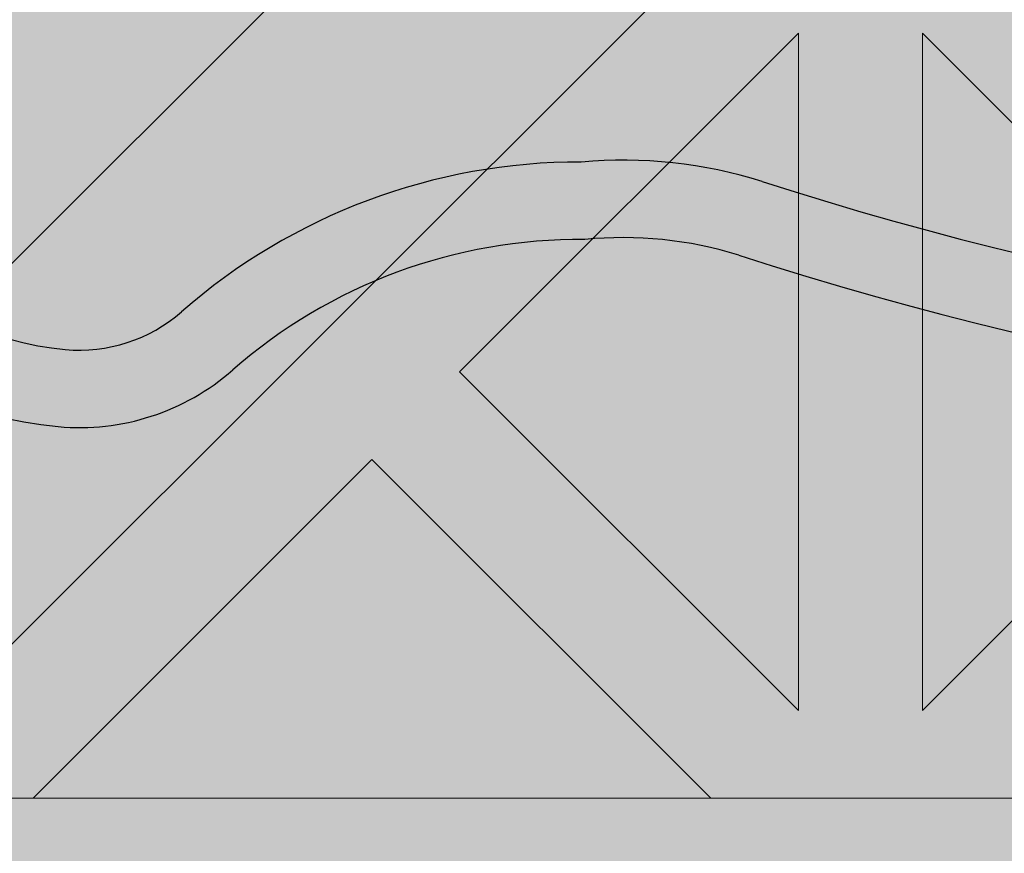
# Model space of a CAD drawing. Units: inches. Extents: x 844 to 2234, y 346 to 1084.
# Tile 10 of 93: x 1119.118 to 1121.143, y 686.542 to 688.258. Entities that reach past the tile are written whole.
import ezdxf

# ---------------------------------------------------------------- set-up
doc = ezdxf.new("R2010")
doc.units = ezdxf.units.IN
doc.header["$MEASUREMENT"] = 0
for name, color, linetype, lineweight in [('A-ANNO-DIMS', 2, 'Continuous', 18), ('furniture', 8, 'Continuous', 18), ('RA-AP-01$0$INT', 35, 'Continuous', 5)]:
    doc.layers.add(name, color=color, linetype=linetype, lineweight=lineweight)
doc.layers.add('RA-AP-01$0$FURN', color=3, linetype='Continuous')
doc.layers.add('RA-AP-01$0$WOOD', color=64, linetype='Continuous')
doc.styles.get("Standard").update_dxf_attribs({"font": 'arial.ttf'})
doc.dimstyles.get("Standard").update_dxf_attribs({"dimtxt": 6, "dimasz": 3, "dimexe": 0.18, "dimexo": 0.0625, "dimgap": 0.09, "dimtad": 0, "dimtih": 1, "dimtoh": 1, "dimdec": 1, "dimzin": 0, "dimdsep": 46, "dimlunit": 3, "dimtxsty": 'Standard', "dimblk": 'ARCHTICK', "dimcen": 0.09, "dimadec": 0, "dimazin": 0, "dimtfac": 1, "dimtdec": 1, "dimtofl": 0, "dimtmove": 0, "dimatfit": 3, "dimfxl": 1, "dimtolj": 1, "dimtzin": 0, "dimarcsym": 0})

# ---------------------------------------------------------------- blocks, each defined once
blk = doc.blocks.new('A$C18D01794')
at = {"layer": 'RA-AP-01$0$INT'}
blk.add_hatch(color=256, dxfattribs=at).paths.add_polyline_path([(4.505206456958071, -6.306712009588038), (5.305206456958072, -6.306712009588038), (5.305206456958072, -7.106712009588038), (5.255206456951893, -7.10671200958804), (5.25520645694868, -6.356712009605972), (4.555206456959269, -6.356712009587461), (4.555206456956052, -7.106712009588038), (4.505206456958073, -7.106712009588038)])
h = blk.add_hatch(color=256, dxfattribs=at)
h.paths.add_polyline_path([(4.585917135068449, -6.356712009588271), (4.555206456959269, -6.35671200958746), (4.555206456959137, -6.387422687716308), (4.874495778835233, -6.706712009592356), (4.90520645695423, -6.676001331474049)])
h.paths.add_polyline_path([(5.255206456948813, -6.387422687716306), (5.255206456948682, -6.356712009605972), (5.224495778822613, -6.356712009605161), (4.905206456953498, -6.676001331474273), (4.935917135072151, -6.706712009592924)])
h.paths.add_polyline_path([(4.935917135072559, -6.706712009592068), (4.905206456953564, -6.737422687710376), (5.255206456951813, -7.087422687708613), (5.255206456951549, -7.026001331471008)])
h.paths.add_polyline_path([(4.555206456956399, -7.026001331471013), (4.555206456956134, -7.087422687708616), (4.905206456953821, -6.737422687710943), (4.874495778835166, -6.70671200959229)])
h = blk.add_hatch(color=256, dxfattribs=at)
h.paths.add_polyline_path([(4.585917135068448, -6.356712009588273), (4.614201406330596, -6.356712009589021), (4.668846067270487, -6.411356670531338), (4.723490728212344, -6.356712009591912), (4.771774999457151, -6.35671200959319), (4.826419660396886, -6.411356670535356), (4.862780050090322, -6.374996280843536), (4.844495778842715, -6.356712009595112), (4.862780050090411, -6.356712009595595), (4.905206456960182, -6.399138416468211), (4.947632863832445, -6.356712009597838), (4.965917135079675, -6.356712009598322), (4.947632863831759, -6.374996280845421), (4.983993253523576, -6.411356670538857), (5.038637914464627, -6.356712009600247), (5.08692218571208, -6.356712009601523), (5.141566846649976, -6.411356670541852), (5.196211507589851, -6.356712009604411), (5.224495778822615, -6.356712009605161), (4.905206456953975, -6.676001331473793)])
h.paths.add_polyline_path([(4.895206456956031, -6.637717060225675), (4.895206456958921, -6.528427738347902), (4.840561796018589, -6.583072399285802)], flags=16)
h.paths.add_polyline_path([(4.915206456955638, -6.637717060226121), (4.969851117895509, -6.583072399288678), (4.915206456957609, -6.528427738348344)], flags=16)
h.paths.add_polyline_path([(4.826419660395175, -6.568930263661755), (4.881064321335613, -6.514285602723745), (4.771774999456703, -6.514285602720857)], flags=16)
h.paths.add_polyline_path([(4.983993253519558, -6.568930263665262), (5.038637914460456, -6.514285602726792), (4.929348592581548, -6.514285602724816)], flags=16)
h.paths.add_polyline_path([(4.881064321336025, -6.494285602723742), (4.826419660397532, -6.439640941782821), (4.771774999457062, -6.494285602720859)], flags=16)
h.paths.add_polyline_path([(4.929348592582019, -6.494285602724817), (5.038637914460982, -6.494285602726792), (4.983993253522945, -6.439640941786327)], flags=16)
h.paths.add_polyline_path([(4.895206456960191, -6.480143467100443), (4.895206456962115, -6.407422687715913), (4.876922185715016, -6.389138416467584), (4.840561796021581, -6.425498806159401)], flags=16)
h.paths.add_polyline_path([(4.915206456958487, -6.480143467100889), (4.969851117899527, -6.425498806162279), (4.933490728206909, -6.389138416468043), (4.9152064569598, -6.40742268771434)], flags=16)
h.paths.add_polyline_path([(4.757632863832376, -6.480143467096812), (4.812277524772842, -6.425498806158772), (4.757632863834348, -6.370854145217844)], flags=16)
h.paths.add_polyline_path([(4.737632863832376, -6.480143467096286), (4.737632863834348, -6.370854145217375), (4.682988202893906, -6.425498806155385)], flags=16)
h.paths.add_polyline_path([(5.05278005008503, -6.480143467103376), (5.052780050087917, -6.370854145224413), (4.998135389146995, -6.425498806162908)], flags=16)
h.paths.add_polyline_path([(5.072780050085024, -6.480143467103744), (5.127424711025931, -6.42549880616527), (5.072780050087916, -6.370854145224832)], flags=16)
h.paths.add_polyline_path([(4.935917135072783, -6.706712009592292), (5.255206456948811, -6.387422687716309), (5.255206456948932, -6.415706958964177), (5.200561796010279, -6.470351619902839), (5.255206456949403, -6.524996280841948), (5.25520645694961, -6.5732805520894), (5.200561796009787, -6.627925213029239), (5.236922185702417, -6.664285602721864), (5.255206456949919, -6.646001331474357), (5.255206456949998, -6.664285602721898), (5.212780050078687, -6.706712009592262), (5.25520645695036, -6.749138416463932), (5.255206456950438, -6.767422687711313), (5.236922185702424, -6.749138416463297), (5.200561796009796, -6.785498806155928), (5.255206456950753, -6.840143467096874), (5.25520645695096, -6.888427738341682), (5.200561796010322, -6.943072399282328), (5.255206456951428, -6.997717060223427), (5.255206456951547, -7.026001331471006)])
h.paths.add_polyline_path([(5.042988202883395, -6.785498806155427), (5.097632863823085, -6.840143467095101), (5.097632863822622, -6.730854145216193)], flags=16)
h.paths.add_polyline_path([(5.028846067259663, -6.771356670531693), (5.083490728198774, -6.716712009592573), (4.974201406321001, -6.716712009593042)], flags=16)
h.paths.add_polyline_path([(5.117632863823087, -6.840143467095186), (5.172277524762331, -6.785498806155926), (5.11763286382262, -6.730854145216225)], flags=16)
h.paths.add_polyline_path([(5.08349072819877, -6.696712009593886), (5.028846067259652, -6.642067348654775), (4.974201406320998, -6.696712009593438)], flags=16)
h.paths.add_polyline_path([(5.131774999446817, -6.854285602718917), (5.186419660386065, -6.799640941779662), (5.241064321325782, -6.854285602719365)], flags=17)
h.paths.add_polyline_path([(5.131774999446228, -6.716712009592374), (5.186419660386065, -6.771356670532194), (5.222780050079488, -6.734996280838764), (5.204495778832781, -6.716712009592063)], flags=16)
h.paths.add_polyline_path([(5.097632863822613, -6.682569873970264), (5.097632863823061, -6.573280552091354), (5.042988202883383, -6.627925213031044)], flags=16)
h.paths.add_polyline_path([(5.131774999446899, -6.874285602718915), (5.241064321325809, -6.874285602719364), (5.186419660386591, -6.928930263658598)], flags=17)
h.paths.add_polyline_path([(5.131774999446226, -6.696712009594078), (5.204495778830767, -6.696712009594374), (5.22278005007868, -6.67842773834687), (5.186419660386049, -6.642067348654249)], flags=16)
h.paths.add_polyline_path([(5.11763286382262, -6.682569873970225), (5.17227752476232, -6.627925213030515), (5.117632863823064, -6.573280552091267)], flags=16)
h.paths.add_polyline_path([(5.186419660386069, -6.613783077405491), (5.241064321325754, -6.559138416465795), (5.131774999446791, -6.559138416466263)], flags=16)
h.paths.add_polyline_path([(5.131774999446872, -6.539138416466263), (5.24106432132578, -6.539138416465794), (5.186419660386554, -6.484493755526573)], flags=16)
h.paths.add_polyline_path([(5.255206456951811, -7.08742268770861), (5.255206456951895, -7.106712009588038), (4.555206456956052, -7.106712009588038), (4.555206456956136, -7.087422687708617), (4.905206456953973, -6.737422687710788)])
h.paths.add_polyline_path([(4.983993253513404, -6.8444937555241), (4.92934859257295, -6.899138416462108), (5.03863791445186, -6.899138416465014)], flags=16)
h.paths.add_polyline_path([(4.969851117889988, -6.83035161990006), (4.915206456952556, -6.775706958960171), (4.915206456949648, -6.884996280837944)], flags=16)
h.paths.add_polyline_path([(4.929348592572535, -6.919138416462105), (4.983993253511019, -6.973783077403037), (5.038637914451496, -6.919138416465012)], flags=16)
h.paths.add_polyline_path([(5.052780050074912, -6.93328055208906), (4.998135389134438, -6.987925213027088), (5.052780050072919, -7.042569873968025)], flags=16)
h.paths.add_polyline_path([(5.07278005007491, -6.933280552089588), (5.072780050072918, -7.042569873968497), (5.127424711013374, -6.987925213030498)], flags=16)
h.paths.add_polyline_path([(4.89520645695295, -6.775706958959721), (4.840561796013067, -6.830351619897157), (4.895206456950961, -6.884996280837494)], flags=16)
h.paths.add_polyline_path([(4.915206456948365, -6.933280552085403), (4.915206456946434, -7.006001331471951), (4.933490728192729, -7.024285602719066), (4.969851117886972, -6.987925213026453)], flags=16)
h.paths.add_polyline_path([(4.881064321327021, -6.899138416461022), (4.82641966038902, -6.84449375552057), (4.771774999448108, -6.899138416459029)], flags=16)
h.paths.add_polyline_path([(4.895206456950073, -6.933280552084951), (4.840561796009022, -6.987925213023558), (4.876922185700835, -7.024285602716997), (4.895206456948749, -7.006001331469487)], flags=16)
h.paths.add_polyline_path([(4.983993253510392, -7.0020673486505), (4.947632863816944, -7.038427738342319), (4.965917135064043, -7.05671200959023), (5.038637914448995, -7.056712009591555)], flags=16)
h.paths.add_polyline_path([(4.881064321326543, -6.91913841646102), (4.771774999447578, -6.919138416459031), (4.826419660385607, -6.973783077399508)], flags=16)
h.paths.add_polyline_path([(4.905206456946447, -7.014285602717636), (4.862780050074785, -7.056712009588352), (4.947632863816685, -7.056712009589775)], flags=16)
h.paths.add_polyline_path([(5.14156684663679, -7.002067348654549), (5.086922185696452, -7.056712009592438), (5.196211507574223, -7.056712009594425)], flags=16)
h.paths.add_polyline_path([(4.8264196603837, -7.002067348646972), (4.771774999442643, -7.056712009585575), (4.8444957788276, -7.056712009587508), (4.862780050075511, -7.038427738340416)], flags=16)
h.paths.add_polyline_path([(4.812277524760289, -6.98792521302292), (4.757632863822258, -6.933280552082447), (4.757632863819352, -7.042569873961408)], flags=16)
h.paths.add_polyline_path([(4.73763286382226, -6.933280552082079), (4.682988202881349, -6.987925213020536), (4.737632863819352, -7.04256987396099)], flags=16)
h.paths.add_polyline_path([(4.723490728195188, -7.056712009584289), (4.668846067257299, -7.002067348643949), (4.614201406317417, -7.056712009581383)], flags=16)
h.paths.add_polyline_path([(4.597632863829262, -6.706712009592262), (4.555206456957951, -6.664285602721896), (4.555206456958029, -6.646001331474357), (4.573490728205535, -6.664285602721864), (4.609851117898167, -6.627925213029238), (4.555206456958338, -6.573280552089402), (4.555206456958546, -6.524996280841952), (4.60985111789767, -6.470351619902839), (4.555206456959015, -6.415706958964177), (4.555206456959138, -6.387422687716309), (4.874495778835167, -6.70671200959229), (4.5552064569564, -7.026001331471015), (4.555206456956523, -6.997717060223433), (4.609851117897629, -6.94307239928233), (4.555206456956988, -6.888427738341681), (4.555206456957198, -6.840143467096881), (4.609851117898153, -6.78549880615593), (4.573490728205528, -6.749138416463297), (4.555206456957507, -6.76742268771132), (4.555206456957585, -6.749138416463933)])
h.paths.add_polyline_path([(4.712780050085332, -6.730854145216195), (4.712780050084863, -6.840143467095105), (4.767424711024555, -6.785498806155427)], flags=16)
h.paths.add_polyline_path([(4.726922185709173, -6.716712009592573), (4.781566846648288, -6.771356670531693), (4.836211507586949, -6.716712009593043)], flags=16)
h.paths.add_polyline_path([(4.692780050085327, -6.730854145216225), (4.638135389145619, -6.785498806155928), (4.692780050084865, -6.840143467095185)], flags=16)
h.paths.add_polyline_path([(4.726922185709182, -6.696712009593886), (4.836211507586949, -6.696712009593436), (4.7815668466483, -6.642067348654773)], flags=16)
h.paths.add_polyline_path([(4.678637914461726, -6.71671200959237), (4.605917135075169, -6.716712009592063), (4.587632863828464, -6.734996280838766), (4.623993253521887, -6.771356670532195)], flags=16)
h.paths.add_polyline_path([(4.712780050085336, -6.68256987397026), (4.767424711024568, -6.627925213031042), (4.71278005008489, -6.573280552091352)], flags=16)
h.paths.add_polyline_path([(4.678637914461726, -6.696712009594076), (4.623993253521899, -6.642067348654247), (4.587632863829271, -6.67842773834687), (4.605917135077185, -6.696712009594376)], flags=16)
h.paths.add_polyline_path([(4.692780050085336, -6.682569873970228), (4.692780050084889, -6.573280552091267), (4.638135389145632, -6.627925213030515)], flags=16)
h.paths.add_polyline_path([(4.623993253521885, -6.799640941779662), (4.678637914461131, -6.854285602718915), (4.56934859258217, -6.854285602719365)], flags=17)
h.paths.add_polyline_path([(4.623993253521901, -6.613783077405509), (4.678637914461158, -6.559138416466263), (4.569348592582195, -6.559138416465795)], flags=16)
h.paths.add_polyline_path([(4.678637914461051, -6.874285602718915), (4.623993253521361, -6.928930263658598), (4.569348592582143, -6.874285602719364)], flags=17)
h.paths.add_polyline_path([(4.678637914461076, -6.539138416466263), (4.623993253521399, -6.484493755526573), (4.569348592582167, -6.539138416465796)], flags=16)
h = blk.add_hatch(color=256, dxfattribs=at)
h.paths.add_polyline_path([(4.969851117891331, -6.583072399286455), (4.915206456952669, -6.63771706022511), (4.915206456952222, -6.528427738347337)])
h.paths.add_polyline_path([(4.895206456953064, -6.637717060225108), (4.840561796014413, -6.583072399286448), (4.895206456953533, -6.528427738347335)])
h.paths.add_polyline_path([(4.826419660390684, -6.568930263662714), (4.771774999451003, -6.514285602723024), (4.881064321329913, -6.514285602723489)])
h.paths.add_polyline_path([(4.881064321329884, -6.494285602723492), (4.771774999450921, -6.494285602723024), (4.82641966039018, -6.439640941783778)])
h.paths.add_polyline_path([(4.895206456953734, -6.48014346709988), (4.840561796013912, -6.425498806160046), (4.876922185707337, -6.389138416466622), (4.895206456954043, -6.40742268771333)])
h.paths.add_polyline_path([(4.862780050082808, -6.374996280843689), (4.826419660390178, -6.411356670536314), (4.771774999450351, -6.356712009596481), (4.844495778835303, -6.356712009596181)])
h.paths.add_polyline_path([(4.812277524766446, -6.425498806160041), (4.757632863827191, -6.480143467099289), (4.757632863826741, -6.370854145220329)])
h.paths.add_polyline_path([(4.737632863827191, -6.480143467099214), (4.682988202887508, -6.425498806159518), (4.737632863826743, -6.370854145220299)])
h.paths.add_polyline_path([(4.668846067263777, -6.41135667053579), (4.614201406325123, -6.356712009597128), (4.723490728202894, -6.356712009596675)])
h.paths.add_polyline_path([(4.905206456953846, -6.399138416467422), (4.862780050082654, -6.356712009596229), (4.947632863824561, -6.356712009595756)])
h.paths.add_polyline_path([(4.915206456952028, -6.480143467099882), (4.91520645695173, -6.407422687715346), (4.933490728199234, -6.389138416467428), (4.96985111789186, -6.425498806160055)])
h.paths.add_polyline_path([(5.038637914454841, -6.494285602723048), (4.929348592575874, -6.494285602723497), (4.983993253515593, -6.439640941783787)])
h.paths.add_polyline_path([(4.983993253515065, -6.568930263662725), (4.929348592575849, -6.514285602723495), (5.038637914454755, -6.514285602723045)])
h.paths.add_polyline_path([(5.052780050079843, -6.480143467099317), (4.998135389140595, -6.425498806160058), (5.052780050080309, -6.370854145220356)])
h.paths.add_polyline_path([(4.983993253516868, -6.411356670536324), (4.947632863824241, -6.374996280843694), (4.965917135071747, -6.356712009596188), (5.038637914456701, -6.356712009596504)])
h.paths.add_polyline_path([(5.127424711019533, -6.425498806159557), (5.072780050079843, -6.480143467099239), (5.07278005008031, -6.370854145220326)])
h.paths.add_polyline_path([(5.141566846643269, -6.411356670535829), (5.086922185704154, -6.356712009596707), (5.196211507581929, -6.356712009597176)])
for p, q in [((4.555206456959269, -6.356712009587461), (5.255206456948681, -6.356712009605972)), ((4.905206456953975, -6.676001331473793), (4.585917135071132, -6.356712009590955)), ((4.614201406333045, -6.356712009591467), (4.668846067270487, -6.41135667053134)), ((4.723490728210815, -6.356712009593442), (4.668846067270487, -6.41135667053134)), ((4.737632863834348, -6.370854145217375), (4.682988202893906, -6.425498806155385)), ((4.737632863832376, -6.480143467096285), (4.737632863834348, -6.370854145217375)), ((4.757632863832376, -6.48014346709681), (4.757632863834348, -6.370854145217847)), ((4.757632863834348, -6.370854145217847), (4.812277524772842, -6.425498806158774)), ((4.874495778835167, -6.70671200959229), (4.555206456959136, -6.387422687716307)), ((4.682988202893908, -6.425498806155387), (4.737632863832376, -6.480143467096285)), ((4.757632863832376, -6.48014346709681), (4.812277524772842, -6.425498806158774))]:
    blk.add_line(p, q, dxfattribs=at)
blk = doc.blocks.new('A$C32926AE1')
at = {"layer": 'RA-AP-01$0$WOOD'}
h = blk.add_hatch(color=256, dxfattribs=at)
h.dxf.hatch_style = 1
h.paths.add_polyline_path([(5.157430609644524, 4.573483066760929, -0.1009492694046607), (5.155401577623758, 4.593365984175333, -0.1842662638101597), (5.172249623284174, 4.638795604568598, 0.2056608120311276), (5.179560981299304, 4.661316324430096, 0.3614336704623542), (5.134352340494423, 4.706524965234944, 0.2056608120311297), (5.111831620632933, 4.699213607219793, -0.1842662638101113), (5.066402000239693, 4.682365561559342, -0.1055311479399994), (5.045656153913092, 4.68467289944697, 0.1567636581983829), (4.763886414745334, 4.684672899446966, -0.1055311479399895), (4.743140568418733, 4.68236556155934, -0.1842662638100833), (4.6977109480255, 4.69921360721979, 0.2056608120302612), (4.675190228164109, 4.706524965234949, 0.3614336704708441), (4.629981587358889, 4.66131632442871, 0.2056608120245944), (4.637292945374126, 4.638795604567974, -0.1842662638101024), (4.654140991034615, 4.59336598417475, -0.1009492694055169), (4.652111959013835, 4.573483066760181, 0.021410119221476), (4.629748025606143, 4.156712009541676, 0.0214101192214795), (4.652111959013809, 3.739940952323101, -0.1009492694059586), (4.654140991034615, 3.720058034908448, -0.1842662638100975), (4.637292945374126, 3.674628414515226, 0.2056608120245705), (4.629981587358889, 3.652107694654492, 0.3614336704708879), (4.675190228164113, 3.606899053848249, 0.2056608120302384), (4.697710948025501, 3.614210411863408, -0.1842662638100995), (4.743140568418738, 3.63105845752386, -0.1055311479402541), (4.763886414745388, 3.628751119636215, 0.1567636581983776), (5.045656153913137, 3.628751119636244, -0.1055311479397538), (5.066402000239692, 3.631058457523857, -0.1842662638101067), (5.111831620632931, 3.614210411863407, 0.2056608120310924), (5.134352340494417, 3.606899053848256, 0.3614336704624001), (5.179560981299307, 3.652107694653103, 0.2056608120311314), (5.172249623284175, 3.6746284145146, -0.1842662638101402), (5.155401577623758, 3.72005803490786, -0.1009492694051366), (5.15743060964455, 3.739940952322354, 0.0214101192215073), (5.179794543052287, 4.156712009541468, 0.0214101192215252)])
h.paths.add_polyline_path([(4.639748609479751, 4.156712009541513, 0.0213537860821624), (4.661970494867118, 3.741887061152232, -0.094075836301374), (4.664143710413708, 3.7196126951003, -0.1824818158568985), (4.644813765429836, 3.668037719127816, 0.2056608120245319), (4.639939526753007, 3.653023905887301, 0.3614336704710246), (4.676106439397173, 3.616856993242342, 0.2056608120302234), (4.691120252638095, 3.621731231919122, -0.1824818158602558), (4.742695228611606, 3.641061176902986, -0.1029891339458722), (4.766991894714349, 3.638256818950944, 0.156709409989566), (5.042550673941472, 3.638256818950105, -0.102989133958497), (5.066847340047078, 3.641061176902949, -0.1824818158594995), (5.118422316020358, 3.621731231919103, 0.2056608120311416), (5.133436129261316, 3.616856993242346, 0.3614336704621468), (5.169603041905217, 3.653023905886178, 0.2056608120310986), (5.164728803228477, 3.668037719127177, -0.1824818158565612), (5.145398858244737, 3.719612695099578, -0.0940758363009313), (5.147572073791232, 3.741887061151398, 0.0213537860822023), (5.169793959178681, 4.156712009541451, 0.0213537860822226), (5.147572073791203, 4.571536957931898, -0.0940758363005034), (5.145398858244737, 4.59381132398362, -0.1824818158565587), (5.164728803228476, 4.645386299956021, 0.2056608120311045), (5.169603041905216, 4.66040011319702, 0.3614336704621845), (5.133436129261313, 4.696567025840856, 0.2056608120310773), (5.118422316020359, 4.691692787164098, -0.182481815859508), (5.066847340047078, 4.67236284218025, -0.1029891339584606), (5.04255067394148, 4.675167200133092, 0.156709409989566), (4.766991894714357, 4.675167200132257, -0.1029891339458842), (4.742695228611611, 4.672362842180213, -0.1824818158602725), (4.691120252638095, 4.691692787164077, 0.2056608120302152), (4.676106439397174, 4.696567025840858, 0.3614336704710363), (4.639939526753005, 4.660400113195899, 0.2056608120245495), (4.644813765429837, 4.645386299955384, -0.1824818158568934), (4.664143710413708, 4.593811323982902, -0.0940758363009187), (4.661970494867149, 4.571536957931074, 0.021353786082177)], flags=16)
h.paths.add_polyline_path([(5.129794543052235, 4.432167055276933, -0.0141661062790638), (5.130152669293814, 4.156927903047693, -0.0141661062790647), (5.129794543052234, 3.881688750818433, -0.0785247771143638), (5.10979738006795, 3.755143611847103, 0.0945969212073497), (5.105408519571111, 3.717898134952927, 0.1043170707844957), (5.116074640131521, 3.670385395016088, 0.1043170707864965), (5.068561900193738, 3.681051515576561, 0.09459692119553), (5.031316423304057, 3.676662655080835, -0.1580239521427272), (4.778226145355827, 3.676662655080367, 0.0945969211986668), (4.740980668464973, 3.681051515576592, 0.1043170707882822), (4.693467928526415, 3.670385395015844, 0.1043170707867916), (4.704134049087309, 3.717898134953662, 0.0945969211972894), (4.69974518859162, 3.755143611844042, -0.0785247771163196), (4.679748025606343, 3.881688750818406, -0.0141661062790663), (4.679389899364763, 4.156927903047693, -0.0141661062790672), (4.679748025606343, 4.432167055276998, -0.0785247771163064), (4.699745188591625, 4.55871219425134, 0.094596921197333), (4.704134049087308, 4.595957671141738, 0.1043170707867205), (4.693467928526416, 4.643470411079523, 0.1043170707882628), (4.740980668464965, 4.632804290518776, 0.0945969211988114), (4.778226145355874, 4.637193151015016, -0.158023952142669), (5.031316423304015, 4.637193151014546, 0.0945969211956361), (5.068561900193736, 4.632804290518806, 0.1043170707864979), (5.11607464013152, 4.643470411079278, 0.1043170707844617), (5.105408519571112, 4.595957671142455, 0.0945969212074597), (5.109797380067959, 4.558712194248236, -0.0785247771143467)], flags=0)
h.paths.add_polyline_path([(5.119794532311105, 4.432259799204851, -0.0142000800617244), (5.120156169157484, 4.156927903047701, -0.0142000800617277), (5.119794532311105, 3.881596006890482, -0.0784894509520253), (5.100273383573699, 3.758192358677797, 0.0940138827242913), (5.095413455884425, 3.717477693979438, 0.0606271852308753), (5.099615656341024, 3.686844378806616, 0.0606271852322524), (5.068982341167493, 3.691046579263239, 0.0940138827010453), (5.028267676478798, 3.686186651576848, -0.1580706864508061), (4.781274892180912, 3.686186651576435, 0.0940138827026903), (4.740560227491556, 3.691046579263279, 0.0606271852339895), (4.709926912317155, 3.686844378806508, 0.0606271852329405), (4.714129112773991, 3.717477693980356, 0.094013882701304), (4.709269185087677, 3.758192358669163, -0.0784894509577193), (4.689748036347473, 3.881596006890469, -0.014200080061729), (4.689386399501094, 4.156927903047709, -0.0142000800617217), (4.689748036347473, 4.432259799204808, -0.078489450957724), (4.709269185087651, 4.555663447426125, 0.0940138827014585), (4.714129112773992, 4.596378112114996, 0.0606271852329731), (4.709926912317154, 4.62701142728886, 0.0606271852340196), (4.74056022749157, 4.622809226832087, 0.0940138827024997), (4.781274892180847, 4.627669154518912, -0.1580706864508359), (5.028267676478777, 4.627669154518526, 0.0940138827010946), (5.068982341167492, 4.622809226832129, 0.060627185232254), (5.099615656341024, 4.627011427288751, 0.0606271852308727), (5.095413455884425, 4.59637811211593, 0.0940138827241088), (5.100273383573675, 4.555663447417647, -0.0784894509520978)], flags=0)
h.paths.add_polyline_path([(5.06978912287499, 4.430218106756144, -0.014241683694547), (5.070173729147532, 4.156927903047672, -0.0142416836945458), (5.06978912287499, 3.883637699339223, -0.0800609523125196), (5.052662118612511, 3.773463122773442, 0.0526421978001116), (5.04590916754064, 3.740550867606997, 0.0526421977992423), (5.012996912374707, 3.73379791653534, -0.1583028414718258), (4.796545656286308, 3.73379791653451, 0.0526421978034211), (4.763633401117837, 3.740550867607021, 0.0526421978018622), (4.756880450045755, 3.773463122774558, -0.0800609523117106), (4.739753445783639, 3.883637699339268, -0.0142416836945435), (4.739368839511098, 4.156927903047671, -0.0142416836945477), (4.739753445783639, 4.430218106756155, -0.0800609523116345), (4.75688045004574, 4.540392683320762, 0.052642197801941), (4.763633401117837, 4.573304938488346, 0.0526421978035071), (4.796545656286361, 4.580057889560873, -0.1583028414717561), (5.012996912374669, 4.580057889560039, 0.0526421977993048), (5.04590916754064, 4.57330493848837, 0.0526421978002057), (5.052662118612529, 4.540392683321868, -0.080060952312477)], flags=0)
h.paths.add_polyline_path([(5.049789715110557, 4.43038092723357, -0.0143097550741839), (5.05018085590259, 4.156927903047715, -0.0143097550741854), (5.049789715110558, 3.883474878861827, -0.0800685599149176), (5.03362098255317, 3.779581877367999, 0.0306258898956367), (5.028241146483733, 3.758218888663947, 0.0306258898977031), (5.006878157778253, 3.75283905259408, -0.1583983521624096), (4.802664410878162, 3.752839052594731, 0.0306258898946014), (4.781301422174808, 3.758218888663924, 0.0306258898967912), (4.775921586105202, 3.779581877368794, -0.080068559914251), (4.759752853548071, 3.883474878861786, -0.0143097550741854), (4.759361712756037, 4.156927903047671, -0.0143097550741854), (4.759752853548071, 4.430380927233557, -0.0800685599142479), (4.775921586105193, 4.534273928726546, 0.0306258898968306), (4.781301422174808, 4.555636917431444, 0.0306258898945754), (4.802664410878143, 4.561016753500631, -0.1583983521624168), (5.006878157778244, 4.561016753501291, 0.0306258898977177), (5.028241146483733, 4.555636917431421, 0.0306258898958182), (5.03362098255321, 4.534273928727244, -0.080068559914796)], flags=0)
h.paths.add_polyline_path([(4.999766070382627, 4.428171244713864, -0.0143443147609634), (5.000198441819402, 4.156927903047689, -0.0143443147609612), (4.999766070382627, 3.885684561381556, -0.0784641635803329), (4.987356730658798, 3.799103304488872, -0.1506053783831347), (4.822185837999821, 3.79910330448882, -0.0784641635803318), (4.809776498276007, 3.885684561381509, -0.014344314760963), (4.809344126839227, 4.156927903047677, -0.0143443147609645), (4.809776498276007, 4.428171244713873, -0.0784641635803192), (4.822185837999822, 4.514752501606549, -0.1506053783831338), (4.987356730658798, 4.514752501606494, -0.078464163580285)], flags=0)
h.paths.add_polyline_path([(4.979755254238824, 4.42764379880488, -0.0143772539198268), (4.980205517789977, 4.156927903047693, -0.0143772539198275), (4.979755254238824, 3.886212007290489, -0.0689242507424422), (4.971183264704897, 3.815276770442801, -0.1296645318904179), (4.838359303953726, 3.815276770442746, -0.0689242507424186), (4.829787314419809, 3.886212007290419, -0.0143772539198292), (4.829337050868653, 4.156927903047653, -0.0143772539198325), (4.829787314419809, 4.427643798804946, -0.0689242507424211), (4.838359303953725, 4.498579035652621, -0.1296645318904187), (4.971183264704897, 4.498579035652565, -0.0689242507424401)], flags=0)
h = blk.add_hatch(color=256, dxfattribs=at)
h.dxf.hatch_style = 1
h.paths.add_polyline_path([(5.145398858244737, 4.59381132398362, -0.1824818158565616), (5.164728803228476, 4.645386299956021, 0.2056608120311045), (5.169603041905216, 4.66040011319702, 0.3614336704621845), (5.133436129261313, 4.696567025840856, 0.2056608120310773), (5.118422316020359, 4.691692787164098, -0.182481815859508), (5.066847340047078, 4.67236284218025, -0.1029891339584606), (5.04255067394148, 4.675167200133092, 0.156709409989566), (4.766991894714357, 4.675167200132257, -0.1029891339458842), (4.742695228611611, 4.672362842180213, -0.1824818158602725), (4.691120252638095, 4.691692787164077, 0.2056608120302152), (4.676106439397174, 4.696567025840858, 0.3614336704710363), (4.639939526753005, 4.660400113195899, 0.2056608120245495), (4.644813765429837, 4.645386299955384, -0.1824818158568934), (4.664143710413708, 4.593811323982902, -0.0940758363009187), (4.661970494867149, 4.571536957931074, 0.0213537860821772), (4.639748609479751, 4.156712009541507, 0.0213537860821625), (4.661970494867119, 3.741887061152226, -0.0940758363013071), (4.664143710413708, 3.719612695100309, -0.1824818158569294), (4.644813765429836, 3.668037719127816, 0.2056608120245319), (4.639939526753007, 3.653023905887301, 0.3614336704710246), (4.676106439397173, 3.616856993242342, 0.2056608120302234), (4.691120252638095, 3.621731231919122, -0.1824818158602558), (4.742695228611606, 3.641061176902986, -0.1029891339458722), (4.766991894714349, 3.638256818950944, 0.156709409989566), (5.042550673941472, 3.638256818950105, -0.102989133958497), (5.066847340047078, 3.641061176902949, -0.1824818158594995), (5.118422316020358, 3.621731231919103, 0.2056608120311416), (5.133436129261316, 3.616856993242346, 0.3614336704621468), (5.169603041905217, 3.653023905886178, 0.2056608120310986), (5.164728803228477, 3.668037719127177, -0.1824818158565612), (5.145398858244737, 3.719612695099578, -0.0940758363009313), (5.147572073791232, 3.741887061151398, 0.0213537860822023), (5.169793959178681, 4.156712009541451, 0.0213537860822226), (5.147572073791203, 4.571536957931898, -0.0940758363004996)])
h.paths.add_polyline_path([(5.109797380067958, 4.55871219424824, -0.0785247771143472), (5.129794543052234, 4.432167055276936, -0.0141661062790644), (5.130152669293814, 4.156927903047685, -0.014166106279066), (5.129794543052234, 3.881688750818401, -0.0785247771143517), (5.109797380067946, 3.755143611847092, 0.0945969212073132), (5.105408519571111, 3.717898134952929, 0.1043170707844995), (5.116074640131521, 3.670385395016088, 0.1043170707864965), (5.068561900193738, 3.681051515576561, 0.09459692119553), (5.031316423304057, 3.676662655080835, -0.1580239521427272), (4.778226145355827, 3.676662655080367, 0.0945969211986668), (4.740980668464973, 3.681051515576592, 0.1043170707882822), (4.693467928526415, 3.670385395015844, 0.1043170707867916), (4.704134049087309, 3.717898134953662, 0.0945969211972894), (4.69974518859162, 3.755143611844042, -0.0785247771163196), (4.679748025606343, 3.881688750818406, -0.0141661062790663), (4.679389899364763, 4.156927903047693, -0.0141661062790672), (4.679748025606343, 4.432167055276998, -0.0785247771163064), (4.699745188591625, 4.55871219425134, 0.094596921197333), (4.704134049087308, 4.595957671141738, 0.1043170707867205), (4.693467928526416, 4.643470411079523, 0.1043170707882628), (4.740980668464965, 4.632804290518776, 0.0945969211988114), (4.778226145355874, 4.637193151015016, -0.158023952142669), (5.031316423304015, 4.637193151014546, 0.0945969211956361), (5.068561900193736, 4.632804290518806, 0.1043170707864979), (5.11607464013152, 4.643470411079278, 0.1043170707844617), (5.105408519571112, 4.595957671142455, 0.0945969212074504)], flags=16)
h.paths.add_polyline_path([(5.100273383573655, 4.55566344741771, -0.0784894509521388), (5.119794532311105, 4.432259799204852, -0.0142000800617252), (5.120156169157484, 4.156927903047686, -0.014200080061726), (5.119794532311105, 3.881596006890502, -0.0784894509520446), (5.100273383573696, 3.758192358677786, 0.0940138827242721), (5.095413455884425, 3.717477693979436, 0.0606271852308692), (5.099615656341024, 3.686844378806616, 0.0606271852322522), (5.068982341167493, 3.691046579263239, 0.0940138827010453), (5.028267676478798, 3.686186651576848, -0.1580706864508061), (4.781274892180912, 3.686186651576435, 0.0940138827026903), (4.740560227491556, 3.691046579263279, 0.0606271852339895), (4.709926912317155, 3.686844378806508, 0.0606271852329405), (4.714129112773991, 3.717477693980356, 0.094013882701304), (4.709269185087677, 3.758192358669163, -0.0784894509577193), (4.689748036347473, 3.881596006890469, -0.014200080061729), (4.689386399501094, 4.156927903047709, -0.0142000800617217), (4.689748036347473, 4.432259799204808, -0.078489450957724), (4.709269185087651, 4.555663447426125, 0.0940138827014585), (4.714129112773992, 4.596378112114996, 0.0606271852329731), (4.709926912317154, 4.62701142728886, 0.0606271852340196), (4.74056022749157, 4.622809226832087, 0.0940138827024997), (4.781274892180847, 4.627669154518912, -0.1580706864508359), (5.028267676478777, 4.627669154518526, 0.0940138827010946), (5.068982341167492, 4.622809226832129, 0.060627185232254), (5.099615656341024, 4.627011427288751, 0.0606271852308727), (5.095413455884425, 4.59637811211593, 0.094013882723957)], flags=0)
h.paths.add_polyline_path([(5.04590916754064, 4.57330493848837, 0.0526421978002057), (5.052662118612529, 4.540392683321868, -0.0800609523124783), (5.06978912287499, 4.430218106756142, -0.0142416836945469), (5.070173729147532, 4.156927903047672, -0.0142416836945458), (5.06978912287499, 3.883637699339223, -0.0800609523125196), (5.052662118612511, 3.773463122773442, 0.0526421978001116), (5.04590916754064, 3.740550867606997, 0.0526421977992423), (5.012996912374707, 3.73379791653534, -0.1583028414718258), (4.796545656286308, 3.73379791653451, 0.0526421978034211), (4.763633401117837, 3.740550867607021, 0.0526421978018622), (4.756880450045755, 3.773463122774558, -0.0800609523117106), (4.739753445783639, 3.883637699339268, -0.0142416836945435), (4.739368839511098, 4.156927903047671, -0.0142416836945477), (4.739753445783639, 4.430218106756155, -0.0800609523116345), (4.75688045004574, 4.540392683320762, 0.052642197801941), (4.763633401117837, 4.573304938488346, 0.0526421978035071), (4.796545656286361, 4.580057889560873, -0.1583028414717561), (5.012996912374669, 4.580057889560039, 0.0526421977993048)], flags=0)
h.paths.add_polyline_path([(5.028241146483733, 4.555636917431422, 0.0306258898956949), (5.033620982553182, 4.534273928727329, -0.0800685599148649), (5.049789715110557, 4.430380927233569, -0.0143097550741839), (5.05018085590259, 4.156927903047715, -0.0143097550741854), (5.049789715110558, 3.883474878861827, -0.0800685599149176), (5.03362098255317, 3.779581877367999, 0.0306258898956367), (5.028241146483733, 3.758218888663947, 0.0306258898977031), (5.006878157778253, 3.75283905259408, -0.1583983521624096), (4.802664410878162, 3.752839052594731, 0.0306258898946014), (4.781301422174808, 3.758218888663924, 0.0306258898967912), (4.775921586105202, 3.779581877368794, -0.080068559914251), (4.759752853548071, 3.883474878861786, -0.0143097550741854), (4.759361712756037, 4.156927903047671, -0.0143097550741854), (4.759752853548071, 4.430380927233557, -0.0800685599142479), (4.775921586105193, 4.534273928726546, 0.0306258898968306), (4.781301422174808, 4.555636917431444, 0.0306258898945754), (4.802664410878143, 4.561016753500631, -0.1583983521624168), (5.006878157778244, 4.561016753501291, 0.0306258898977174)], flags=0)
h.paths.add_polyline_path([(4.987356730658798, 4.514752501606494, -0.0784641635803018), (4.999766070382627, 4.428171244713845, -0.0143443147609637), (5.000198441819402, 4.156927903047665, -0.0143443147609622), (4.999766070382628, 3.885684561381514, -0.0784641635802952), (4.987356730658797, 3.799103304488872, -0.1506053783831338), (4.822185837999821, 3.799103304488819, -0.0784641635803342), (4.809776498276007, 3.885684561381512, -0.0143443147609628), (4.809344126839227, 4.156927903047676, -0.0143443147609646), (4.809776498276007, 4.428171244713873, -0.0784641635803192), (4.822185837999822, 4.514752501606549, -0.1506053783831338)], flags=0)
h.paths.add_polyline_path([(4.971183264704897, 4.498579035652566, -0.0689242507424384), (4.979755254238824, 4.427643798804883, -0.0143772539198276), (4.980205517789977, 4.15692790304768, -0.0143772539198258), (4.979755254238823, 3.88621200729051, -0.0689242507424628), (4.971183264704897, 3.815276770442801, -0.129664531890417), (4.838359303953726, 3.815276770442746, -0.0689242507424186), (4.829787314419809, 3.886212007290419, -0.0143772539198292), (4.829337050868653, 4.156927903047653, -0.0143772539198325), (4.829787314419809, 4.427643798804946, -0.0689242507424211), (4.838359303953725, 4.498579035652621, -0.1296645318904187)], flags=0)
h = blk.add_hatch(dxfattribs=at)
h.set_pattern_fill('ANSI31', color=256, scale=0.05, style=0)
h.set_pattern_definition([(45, (0, 0), (-0.0044194173824159, 0.0044194173824159), [])])
h.paths.add_polyline_path([(5.130152669293814, 4.156927903047704, 0.0141661062790657), (5.129794543052234, 4.432167055276982, 0.0777827904001433), (5.110168979996553, 4.557559993161921, -0.0976515123401879), (5.105408519571111, 4.595957671142454, -0.1043170707844687), (5.116074640131522, 4.64347041107928), (5.099615656341024, 4.627011427288751, 0.0606271852308727), (5.095413455884425, 4.59637811211593, 0.0940138827241088), (5.100273383573675, 4.555663447417647, -0.0784894509520972), (5.119794532311105, 4.432259799204852, -0.0142000800617252), (5.120156169157484, 4.156927903047686, -0.014200080061726), (5.119794532311105, 3.881596006890502, -0.0784894509520446), (5.100273383573696, 3.758192358677786, 0.0940138827242721), (5.095413455884425, 3.717477693979436, 0.0606271852308692), (5.099615656341024, 3.686844378806616), (5.116074640131519, 3.67038539501609, -0.1043170707844594), (5.105408519571112, 3.717898134952912, -0.0976515123401594), (5.11016897999655, 3.756295812933435, 0.0777827904001654), (5.129794543052234, 3.881688750818409, 0.0141661062790665)])
h.paths.add_polyline_path([(5.030164222210597, 3.676291055149937, -0.0976515123472002), (5.068561900193739, 3.681051515576561, -0.1043170707864927), (5.116074640131521, 3.670385395016088), (5.099615656341024, 3.686844378806616, 0.0606271852322522), (5.068982341167493, 3.691046579263239, 0.0940138827010453), (5.028267676478798, 3.686186651576848, -0.1580706864508061), (4.781274892180912, 3.686186651576435, 0.0940138827026903), (4.740560227491556, 3.691046579263279, 0.0606271852339913), (4.709926912317154, 3.686844378806508), (4.693467928526416, 3.670385395015845, -0.1043170707882796), (4.740980668464973, 3.681051515576592, -0.0976515123427246), (4.779378346446416, 3.676291055150394, 0.156512506893803)])
h.paths.add_polyline_path([(4.689748036347473, 3.881596006890472, -0.014200080061729), (4.689386399501094, 4.156927903047712, -0.0142000800617195), (4.689748036347473, 4.432259799204768, -0.078489450957742), (4.709269185087648, 4.555663447426114, 0.0940138827014821), (4.714129112773992, 4.596378112114995, 0.0606271852329748), (4.709926912317154, 4.62701142728886), (4.693467928526414, 4.643470411079524, -0.1043170707867939), (4.704134049087309, 4.595957671141706, -0.09765151234893), (4.699373588660725, 4.557559993157876, 0.0777827903975372), (4.679748025606343, 4.432167055276987, 0.0141661062790675), (4.679389899364763, 4.156927903047675, 0.0141661062790641), (4.679748025606343, 3.88168875081843, 0.0777827903975637), (4.699373588660724, 3.756295812937497, -0.0976515123490278), (4.704134049087308, 3.717898134953629, -0.1043170707867196), (4.693467928526416, 3.670385395015845), (4.709926912317155, 3.686844378806508, 0.0606271852329413), (4.714129112773991, 3.717477693980357, 0.0940138827013084), (4.709269185087676, 3.758192358669166, -0.0784894509577192)])
h.paths.add_polyline_path([(4.779378346446434, 4.63756475094498, -0.0976515123427943), (4.740980668464964, 4.632804290518776, -0.1043170707882609), (4.693467928526416, 4.643470411079523), (4.709926912317154, 4.62701142728886, 0.0606271852340196), (4.74056022749157, 4.622809226832087, 0.0940138827024997), (4.781274892180847, 4.627669154518912, -0.1580706864508359), (5.028267676478777, 4.627669154518526, 0.0940138827010946), (5.068982341167492, 4.622809226832129, 0.060627185232254), (5.099615656341024, 4.627011427288751), (5.116074640131521, 4.643470411079279, -0.1043170707865022), (5.068561900193735, 4.632804290518806, -0.0976515123475899), (5.030164222210446, 4.637564750945479, 0.1565125068936924)])
for centre, radius, start, end in [((4.904771284329219, 4.067062675376636), 0.4103971832811756, 252.0403002450644, 287.9596997551364), ((4.679771284329334, 3.656688750818591), 0.0399999999998732, 185.2568759935751, 264.7431240055498), ((4.679771284329349, 3.656688750818605), 0.0499999999998892, 185.2568759935945, 264.7431240055689), ((4.742507915094546, 3.56309138593928), 0.0779700159630463, 89.86235369886275, 131.2289490796796), ((4.748108354051293, 3.581305858537387), 0.0599999999999989, 72.59387295230013, 95.17619216014101), ((4.904771284329217, 4.067062675376635), 0.4503971832811742, 252.0623235132636, 287.9376764870612), ((4.742507915094499, 3.563091385939265), 0.0679700159630274, 89.46669294863285, 131.2289490796463), ((4.748108354051358, 3.58130585853739), 0.0500000000000024, 72.64431602474727, 95.70207076536123), ((4.904771284329219, 4.067062675376637), 0.4603971832811766, 252.0683908477148, 287.9316091522846), ((4.67793886186326, 3.636772872030528), 0.0199999999999984, 264.7431240057181, 311.2289490796426), ((4.67793886186326, 3.636772872030529), 0.0299999999999992, 264.7431240057202, 311.2289490796434)]:
    blk.add_arc(centre, radius, start, end, dxfattribs=at)
blk = doc.blocks.new('A$C5D2F253E')
at = {"layer": 'RA-AP-01$0$FURN', "xscale": -0.7999999999883585, "yscale": 0.7999999999883585, "zscale": 0.8, "rotation": 90}
blk.add_blockref('A$C18D01794', (-5.687757199772477, 4.75791982714071), dxfattribs=at)
at = {"layer": 'RA-AP-01$0$WOOD', "rotation": 270}
blk.add_blockref('A$C32926AE1', (-4.161339601644158, 5.73852594588169), dxfattribs=at)
blk = doc.blocks.new('_ArchTick')
at = {"color": 0, "linetype": 'ByBlock', "const_width": 0.15}
blk.add_lwpolyline([(-0.5, -0.5), (0.5, 0.5)], dxfattribs=at)
blk = doc.blocks.new('*D144')
at = {"layer": 'A-ANNO-DIMS', "color": 0, "lineweight": -2, "transparency": 16777216}
for p, q in [((1096.615948, 439.3732739999999), (1096.615948, 1074.743301)), ((1143.115948, 492.373274), (1143.115948, 1074.743301)), ((1096.615948, 1074.563301), (1102.481950728513, 1074.563301)), ((1143.115948, 1074.563301), (1137.249945271487, 1074.563301))]:
    blk.add_line(p, q, dxfattribs=at)
at = {"layer": 'Defpoints', "color": 0, "transparency": 16777216}
for p in [(1143.115948, 1074.563301), (1143.115948, 492.3107739999999), (1096.615948, 439.3107739999999)]:
    blk.add_point(p, dxfattribs=at)
at = {"layer": 'A-ANNO-DIMS', "color": 0, "lineweight": -2, "transparency": 16777216, "xscale": 3, "yscale": 3, "zscale": 3, "rotation": 180}
blk.add_blockref('_ArchTick', (1096.615948, 1074.563301), dxfattribs=at)
at = {"layer": 'A-ANNO-DIMS', "color": 0, "lineweight": -2, "transparency": 16777216, "xscale": 3, "yscale": 3, "zscale": 3}
blk.add_blockref('_ArchTick', (1143.115948, 1074.563301), dxfattribs=at)
at = {"layer": 'A-ANNO-DIMS', "color": 0, "transparency": 16777216, "insert": (1119.865948, 1074.563301), "char_height": 6, "attachment_point": 5}
blk.add_mtext('\\A1;3\'-10 1/2"', dxfattribs=at)

msp = doc.modelspace()

# ---------------------------------------------------------------- block references
at = {"layer": 'furniture', "xscale": 15.94108302203742, "yscale": 15.94108302203742, "zscale": 15.94108302203742, "rotation": 90}
msp.add_blockref('A$C5D2F253E', (1136.147844094663, 696.2584716700112), dxfattribs=at)

# ---------------------------------------------------------------- dimensions: what is measured, and where the dimension line sits
at = {"layer": 'A-ANNO-DIMS'}
dim = msp.add_linear_dim(base=(1143.115948, 1074.563301), p1=(1096.615948, 439.3107739999999), p2=(1143.115948, 492.3107739999999), dimstyle='Standard', override={"dimdec": 1, "dimlfac": 1, "dimrnd": 0, "dimzin": 1, "dimdsep": 46, "dimlunit": 4, "dimfrac": 2}, dxfattribs=at)
dim.commit()
dim.dimension.update_dxf_attribs({"geometry": '*D144', "text_midpoint": (1119.865948, 1074.563301)})

doc.saveas('drawing.dxf')
